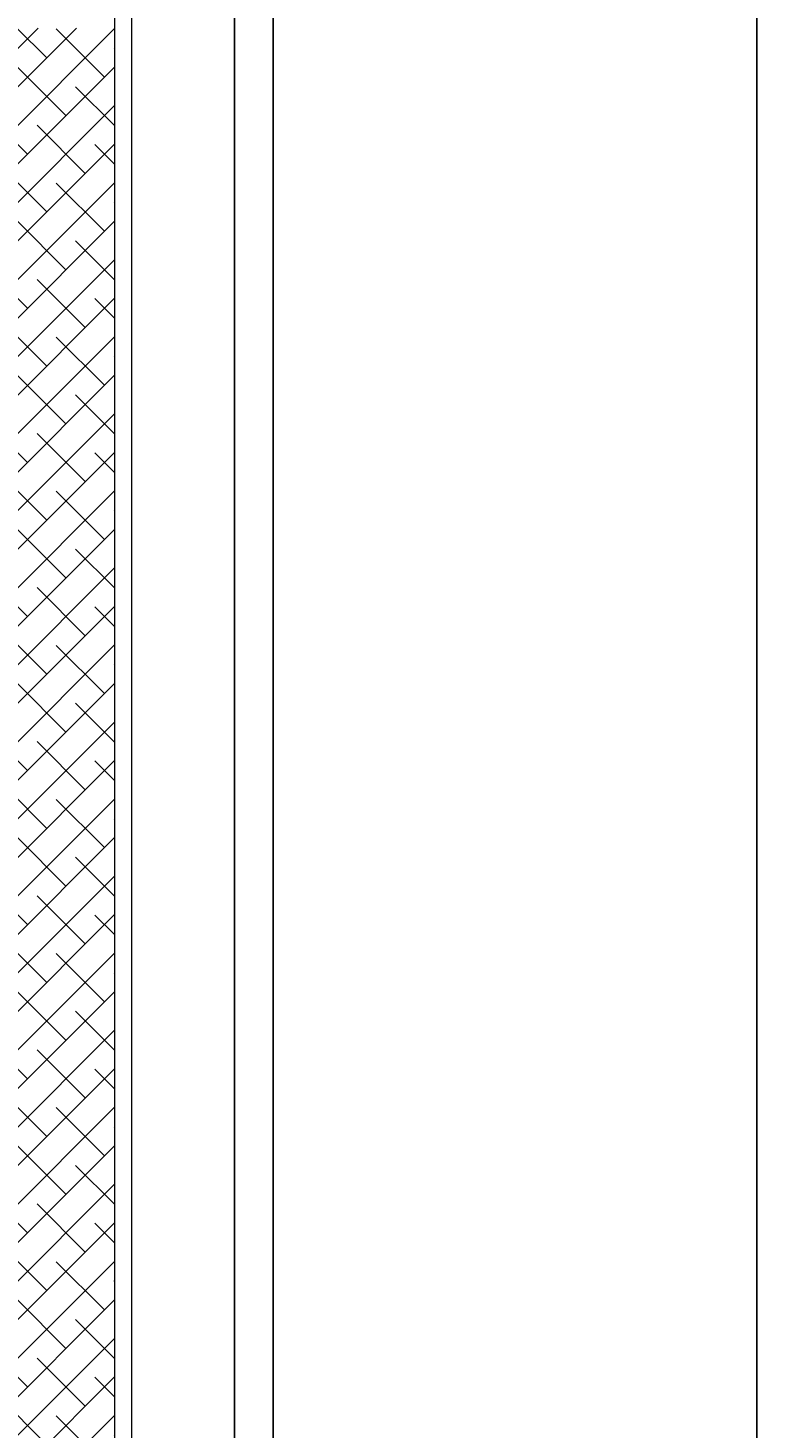
# Model space of a CAD drawing. Units: inches. Extents: x -4843 to -3402, y -164 to 3629.
# Tile 5 of 22: x -3999 to -3829, y 131 to 457. Entities that reach past the tile are written whole.
import ezdxf

# ---------------------------------------------------------------- set-up
doc = ezdxf.new("R2010")
doc.units = ezdxf.units.IN
for name, color, linetype, lineweight in [('A-ANNO-DIMS', 2, 'Continuous', 18), ('C-PROP', 7, 'Continuous', 25), ('L-PLNT-EDGE', 7, 'Continuous', 18)]:
    doc.layers.add(name, color=color, linetype=linetype, lineweight=lineweight)
doc.layers.add('C-PVMT-PATT', color=9, linetype='Continuous', lineweight=13, true_color=0xc7c8ca)
doc.styles.get("Standard").update_dxf_attribs({"font": 'arial.ttf'})
doc.dimstyles.get("Standard").update_dxf_attribs({"dimtxt": 0.18, "dimasz": 0.18, "dimexe": 0.18, "dimexo": 0.0625, "dimgap": 0.09, "dimtad": 0, "dimtih": 1, "dimtoh": 1, "dimdec": 4, "dimzin": 0, "dimdsep": 46, "dimtxsty": 'Standard', "dimcen": 0.09, "dimadec": 0, "dimazin": 0, "dimtfac": 1, "dimtdec": 4, "dimtofl": 0, "dimtmove": 0, "dimatfit": 3, "dimfxl": 1, "dimtolj": 1, "dimtzin": 0, "dimarcsym": 0})

# ---------------------------------------------------------------- blocks, each defined once
blk = doc.blocks.new('*D61')
at = {"layer": 'A-ANNO-DIMS', "color": 0, "lineweight": -2, "transparency": 16777216}
for p, q in [((-3941.72, 1149.35), (-3828.78, 1149.35)), ((-3828.96, 1149.17), (-3828.96, 618.04)), ((-3828.96, 86.53), (-3828.96, 617.67)), ((-3941.72, 86.35), (-3828.78, 86.35))]:
    blk.add_line(p, q, dxfattribs=at)
at = {"layer": 'A-ANNO-DIMS', "color": 0, "transparency": 16777216}
for points in [[(-3828.99, 1149.17), (-3828.93, 1149.17), (-3828.96, 1149.35)], [(-3828.99, 86.53), (-3828.93, 86.53), (-3828.96, 86.35)]]:
    blk.add_solid(points, dxfattribs=at)
at = {"layer": 'Defpoints', "color": 0, "transparency": 16777216}
for p in [(-3941.78, 1149.35), (-3828.96, 1149.35), (-3941.78, 86.35)]:
    blk.add_point(p, dxfattribs=at)
at = {"layer": 'A-ANNO-DIMS', "color": 0, "transparency": 16777216, "insert": (-3828.96, 617.85), "char_height": 0.18, "attachment_point": 5}
blk.add_mtext('\\A1;1063', dxfattribs=at)
blk = doc.blocks.new('*D66')
at = {"layer": 'A-ANNO-DIMS', "color": 0, "lineweight": -2, "transparency": 16777216}
for p, q in [((-4083.78, 457.29), (-4083.78, 10.92)), ((-3941.78, 86.29), (-3941.78, 10.92)), ((-4083.6, 11.1), (-4013.06, 11.1)), ((-3941.96, 11.1), (-4012.5, 11.1))]:
    blk.add_line(p, q, dxfattribs=at)
at = {"layer": 'A-ANNO-DIMS', "color": 0, "transparency": 16777216}
for points in [[(-4083.6, 11.13), (-4083.6, 11.07), (-4083.78, 11.1)], [(-3941.96, 11.13), (-3941.96, 11.07), (-3941.78, 11.1)]]:
    blk.add_solid(points, dxfattribs=at)
at = {"layer": 'Defpoints', "color": 0, "transparency": 16777216}
for p in [(-4083.78, 457.35), (-3941.78, 86.35), (-3941.78, 11.1)]:
    blk.add_point(p, dxfattribs=at)
at = {"layer": 'A-ANNO-DIMS', "color": 0, "transparency": 16777216, "insert": (-4012.78, 11.1), "char_height": 0.18, "attachment_point": 5}
blk.add_mtext('\\A1;142', dxfattribs=at)

msp = doc.modelspace()

# ---------------------------------------------------------------- hatches: boundary and pattern name
at = {"layer": 'C-PVMT-PATT'}
h = msp.add_hatch(dxfattribs=at)
h.set_pattern_fill('ANSI38', color=256, scale=2)
h.set_pattern_definition([(45, (-7766.296, -1992.247), (-4.490128, 4.490128), []), (135, (-7766.296, -1992.247), (-13.470384, 4.490128), [15.875, -9.525])])
h.paths.add_polyline_path([(-4583.98, 275.35), (-4595.78, 275.35), (-4595.78, 324.35), (-4595.78, 373.35), (-4595.78, 466.35), (-4696.78, 466.35), (-4696.78, 95.35), (-4583.98, 95.35), (-4583.98, 226.6)])
h.paths.add_polyline_path([(-4302.78, 226.6), (-4583.98, 226.6), (-4583.98, 95.35), (-4332.78, 95.35), (-4332.78, 86.35), (-4003.68, 86.35), (-4003.68, 95.35), (-3978.78, 95.35), (-3978.78, 457.35), (-4003.68, 457.35), (-4003.68, 139.54), (-4302.78, 139.54)])

# ---------------------------------------------------------------- linework, layer by layer
at = {"layer": 'C-PROP'}
for p, q in [((-3941.78, 1149.35), (-3941.78, 86.35)), ((-3950.78, 1140.35), (-3950.78, 95.35))]:
    msp.add_line(p, q, dxfattribs=at)
at = {"layer": 'L-PLNT-EDGE'}
for p, q in [((-3974.78, 1116.35), (-3974.78, 95.35)), ((-3978.78, 1112.35), (-3978.78, 95.35))]:
    msp.add_line(p, q, dxfattribs=at)

# ---------------------------------------------------------------- dimensions: what is measured, and where the dimension line sits
at = {"layer": 'A-ANNO-DIMS'}
dim = msp.add_linear_dim(base=(-3828.96, 1149.35), p1=(-3941.78, 86.35), p2=(-3941.78, 1149.35), angle=90, dimstyle='Standard', override={"dimdec": 0, "dimlfac": 1, "dimrnd": 0, "dimzin": 0, "dimdsep": 46, "dimlunit": 2}, dxfattribs=at)
dim.commit()
dim.dimension.update_dxf_attribs({"geometry": '*D61', "text_midpoint": (-3828.96, 617.85)})
dim = msp.add_linear_dim(base=(-3941.78, 11.1), p1=(-4083.78, 457.35), p2=(-3941.78, 86.35), dimstyle='Standard', override={"dimdec": 0, "dimlfac": 1, "dimrnd": 0, "dimzin": 0, "dimdsep": 46, "dimlunit": 2}, dxfattribs=at)
dim.commit()
dim.dimension.update_dxf_attribs({"geometry": '*D66', "text_midpoint": (-4012.78, 11.1)})

doc.saveas('drawing.dxf')
